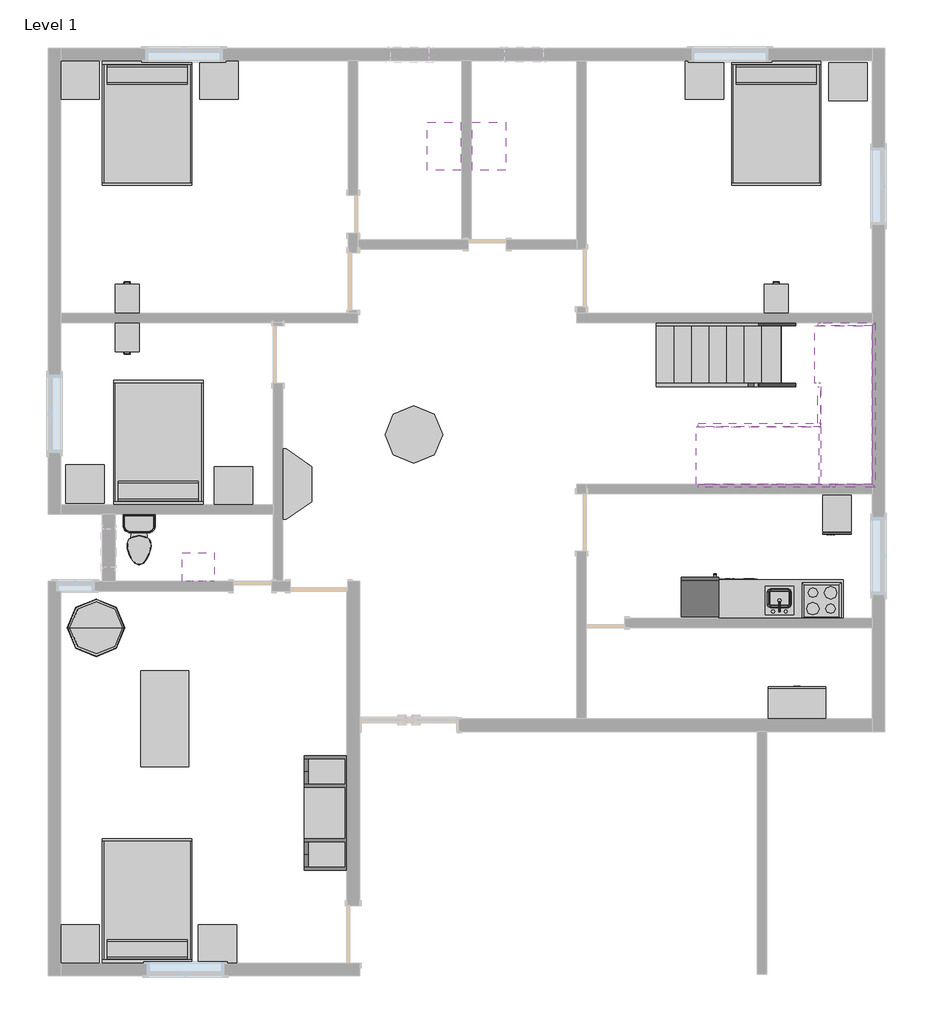
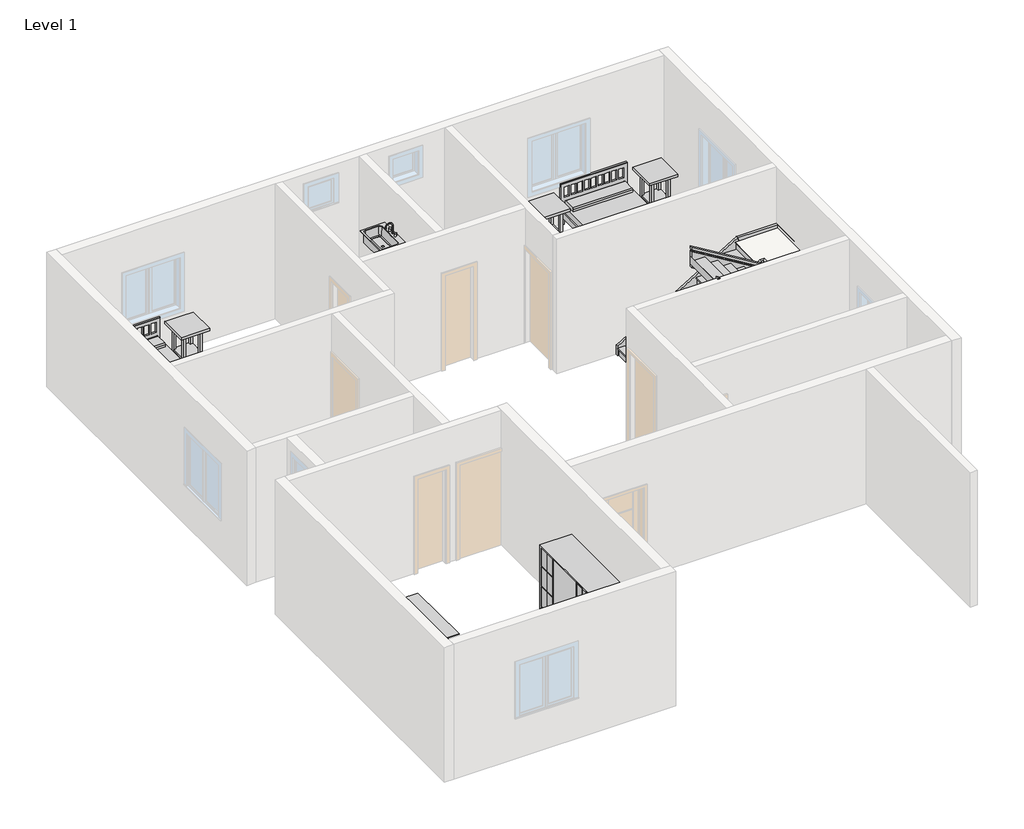
# One storey, part 2 of 2: 22 furniture elements, 8 members, 5 flow terminals, 5 proxies, 2 stair flights, 1 railing, 1 slab.
"""IFC4 building model written with IfcOpenShell, lengths in millimetres."""

from ifc_helpers import new_model, si_unit, frame, origin, place, context, project, spatial, polyline, outline, extrude, faceted_brep, transform, mapped, element, save
from components import proxy_7e1014cc, proxy_a6faaae8, proxy_45b28599, kitchenette_medium_kitchenette_medium_844211aa, proxy_c523a7b7, flow_terminal_98dee406, flow_terminal_871c2e40, flow_terminal_38af2918, toilet_domestic_3d_toilet_domestic_3d_f7549cf7, toilet_domestic_3d_toilet_domestic_3d_183bbd19, furniture_096e7f55, furniture_bb55ed6b, furniture_552c1472, furniture_c6510c7c, furniture_cf0b6580, furniture_e1dba61b, tv_stand_tv_stand_6ce107e5, furniture_37c8c8f5, furniture_905aceb5, furniture_5bc9ed15, furniture_c80d6d9c, non_monolithic_landing_c967b2c0, stair_flight_b85e79d8, stair_flight_81020766

model = new_model("IFC4")

# Units and contexts
model_context = context("Model", 3, world=origin())
ifc_project = project(units=[si_unit("LENGTHUNIT", "METRE", prefix="MILLI")], contexts=[model_context])

# Site, building, storey
site = spatial("IfcSite", under=ifc_project)
building = spatial("IfcBuilding", under=site)
storey = spatial("IfcBuildingStorey", under=building, Name="Level 1", Elevation=0.0)

# Proxies
placement = place(None, origin())
proxy_shape = proxy_7e1014cc(model_context)
element("IfcBuildingElementProxy", 1, Name="18\" x 24\" x 34 1/2\"", ObjectType="18\" x 24\" x 34 1/2\"", at=placement, inside=storey, context=model_context, shape_type="MappedRepresentation", body=[
    mapped(proxy_shape, transform((-3952.7899776, 8163.0653578, 0.0), x_axis=(1.0, 0.0, 0.0), y_axis=(0.0, 1.0, 0.0), z_axis=(0.0, 0.0, 1.0))),
])
proxy_2_shape = proxy_a6faaae8(model_context)
element("IfcBuildingElementProxy", 2, Name="Cook Top-4 Unit2 : 22\" x 20\"", ObjectType="Cook Top-4 Unit2 : 22\" x 20\"", at=placement, inside=storey, context=model_context, shape_type="MappedRepresentation", body=[
    mapped(proxy_2_shape, transform((-3887.9725091, 7057.9149226, 0.0), x_axis=(-1.0000000000000002, 0.0, 0.0), y_axis=(0.0, -1.0000000000000002, 0.0), z_axis=(0.0, 0.0, 1.0))),
])
proxy_3_shape = proxy_45b28599(model_context)
element("IfcBuildingElementProxy", 3, Name="Dishwasher : 24\" x 24\" x 34\"", ObjectType="Dishwasher : 24\" x 24\" x 34\"", at=placement, inside=storey, context=model_context, shape_type="MappedRepresentation", body=[
    mapped(proxy_3_shape, transform((-4839.1550406, 7349.7644874, 0.0), x_axis=(-1.0000000000000002, 0.0, 0.0), y_axis=(0.0, -1.0000000000000002, 0.0), z_axis=(0.0, 0.0, 1.0))),
])
kitchenette_medium_kitchenette_medium_shape = kitchenette_medium_kitchenette_medium_844211aa(model_context)
element("IfcBuildingElementProxy", 4, Name="Kitchenette - Medium : Kitchenette - Medium", ObjectType="Kitchenette - Medium : Kitchenette - Medium", at=placement, inside=storey, context=model_context, shape_type="MappedRepresentation", body=[
    mapped(kitchenette_medium_kitchenette_medium_shape, transform((-4212.1348042, 6753.1149226, 0.0), x_axis=(-1.0000000000000002, 0.0, 0.0), y_axis=(0.0, -1.0000000000000002, 0.0), z_axis=(0.0, 0.0, 1.0))),
])
proxy_4_shape = proxy_c523a7b7(model_context)
element("IfcBuildingElementProxy", 5, Name="Refrigerator : 24\" x 25\" LH", ObjectType="Refrigerator : 24\" x 25\" LH", at=placement, inside=storey, context=model_context, shape_type="MappedRepresentation", body=[
    mapped(proxy_4_shape, transform((-5824.7225091, 7103.5638941, 0.0), x_axis=(-1.0000000000000002, 0.0, 0.0), y_axis=(0.0, -1.0000000000000002, 0.0), z_axis=(0.0, 0.0, 1.0))),
])

# Flow terminals
flow_terminal_shape = flow_terminal_98dee406(model_context)
element("IfcFlowTerminal", 6, ObjectType="Sink - Work : 20\"x18\"", at=placement, inside=storey, context=model_context, shape_type="MappedRepresentation", body=[
    mapped(flow_terminal_shape, transform((-13806.6725091, 7362.7149226, 1524.0), x_axis=(-1.0000000000000004, 0.0, 0.0), y_axis=(0.0, -1.0000000000000004, 0.0), z_axis=(0.0, 0.0, 1.0))),
])
flow_terminal_2_shape = flow_terminal_871c2e40(model_context)
element("IfcFlowTerminal", 7, ObjectType="Sink Kitchen-Island : 18\" x 18\"", at=placement, inside=storey, context=model_context, shape_type="MappedRepresentation", body=[
    mapped(flow_terminal_2_shape, transform((-4545.3832686, 7060.2603237, -14.4), x_axis=(-1.0000000000000002, 0.0, 0.0), y_axis=(0.0, -1.0000000000000002, 0.0), z_axis=(0.0, 0.0, 1.0))),
])
flow_terminal_3_shape = flow_terminal_38af2918(model_context)
element("IfcFlowTerminal", 8, ObjectType="Sink Kitchen-Single : 30\" x 21\"", at=placement, inside=storey, context=model_context, shape_type="MappedRepresentation", body=[
    mapped(flow_terminal_3_shape, transform((-9897.4179102, 14299.9041632, 1219.2), x_axis=(0.0, -1.0000000000000007, 0.0), y_axis=(1.0000000000000007, 0.0, 0.0), z_axis=(0.0, 0.0, 1.0))),
])
element("IfcFlowTerminal", 9, ObjectType="Sink Kitchen-Single : 30\" x 21\"", at=placement, inside=storey, context=model_context, shape_type="MappedRepresentation", body=[
    mapped(flow_terminal_3_shape, transform((-9181.527108, 14268.5256821, 1219.2), x_axis=(0.0, 1.0, 0.0), y_axis=(-1.0, 0.0, 0.0), z_axis=(0.0, 0.0, 1.0))),
])
toilet_domestic_3d_toilet_domestic_3d_shape = toilet_domestic_3d_toilet_domestic_3d_f7549cf7(model_context)
toilet_domestic_3d_toilet_domestic_3d_2_shape = toilet_domestic_3d_toilet_domestic_3d_183bbd19(model_context)
element("IfcFlowTerminal", 10, ObjectType="Toilet-Domestic-3D : Toilet-Domestic-3D", at=placement, inside=storey, context=model_context, shape_type="MappedRepresentation", body=[
    mapped(toilet_domestic_3d_toilet_domestic_3d_shape, transform((-14746.4725091, 7934.8188953, 0.0), x_axis=(1.0, 0.0, 0.0), y_axis=(0.0, 1.0, 0.0), z_axis=(0.0, 0.0, 1.0))),
    mapped(toilet_domestic_3d_toilet_domestic_3d_2_shape, transform((-14746.4725091, 7934.8188953, 0.0), x_axis=(1.0, 0.0, 0.0), y_axis=(0.0, 1.0, 0.0), z_axis=(0.0, 0.0, 1.0))),
])

# Furniture
furniture_shape = furniture_096e7f55(model_context)
element("IfcFurniture", 11, ObjectType="Bed-Shaker : Double 56\" x 78\"", at=placement, inside=storey, context=model_context, shape_type="MappedRepresentation", body=[
    mapped(furniture_shape, transform((-4592.8225091, 15643.1149226, 0.0), x_axis=(1.0, 0.0, 0.0), y_axis=(0.0, 1.0, 0.0), z_axis=(0.0, 0.0, 1.0))),
])
element("IfcFurniture", 12, ObjectType="Bed-Shaker : Double 56\" x 78\"", at=placement, inside=storey, context=model_context, shape_type="MappedRepresentation", body=[
    mapped(furniture_shape, transform((-14600.4225091, 15643.1149226, 0.0), x_axis=(1.0, 0.0, 0.0), y_axis=(0.0, 1.0, 0.0), z_axis=(0.0, 0.0, 1.0))),
])
element("IfcFurniture", 13, ObjectType="Bed-Shaker : Double 56\" x 78\"", at=placement, inside=storey, context=model_context, shape_type="MappedRepresentation", body=[
    mapped(furniture_shape, transform((-14460.7225091, 8581.9149226, 0.0), x_axis=(-1.0, 0.0, 0.0), y_axis=(0.0, -1.0, 0.0), z_axis=(0.0, 0.0, 1.0))),
])
element("IfcFurniture", 14, ObjectType="Bed-Shaker : Double 56\" x 78\"", at=placement, inside=storey, context=model_context, shape_type="MappedRepresentation", body=[
    mapped(furniture_shape, transform((-14638.5225091, 1292.1149226, 0.0), x_axis=(-1.0, 0.0, 0.0), y_axis=(0.0, -1.0, 0.0), z_axis=(0.0, 0.0, 1.0))),
])
furniture_2_shape = furniture_bb55ed6b(model_context)
element("IfcFurniture", 15, ObjectType="Cabinet-File 2 Drawer : 15\" x 18\"", at=placement, inside=storey, context=model_context, shape_type="MappedRepresentation", body=[
    mapped(furniture_2_shape, transform((-14809.0760621, 11391.0492228, 0.0), x_axis=(1.0, 0.0, 0.0), y_axis=(0.0, 1.0, 0.0), z_axis=(0.0, 0.0, 1.0))),
])
furniture_3_shape = furniture_552c1472(model_context)
element("IfcFurniture", 16, ObjectType="Cabinet-File 3 Drawer : 15\" x 18\"", at=placement, inside=storey, context=model_context, shape_type="MappedRepresentation", body=[
    mapped(furniture_3_shape, transform((-15064.8689562, 11716.3806225, 0.0), x_axis=(-1.0000000000000004, 0.0, 0.0), y_axis=(0.0, -1.0000000000000004, 0.0), z_axis=(0.0, 0.0, 1.0))),
])
element("IfcFurniture", 17, ObjectType="Cabinet-File 3 Drawer : 15\" x 18\"", at=placement, inside=storey, context=model_context, shape_type="MappedRepresentation", body=[
    mapped(furniture_3_shape, transform((-4739.7689562, 11716.3806225, 0.0), x_axis=(-1.0000000000000004, 0.0, 0.0), y_axis=(0.0, -1.0000000000000004, 0.0), z_axis=(0.0, 0.0, 1.0))),
])
furniture_4_shape = furniture_c6510c7c(model_context)
element("IfcFurniture", 18, ObjectType="Counter Top w Sink Hole : 24\" Depth", at=placement, inside=storey, context=model_context, shape_type="MappedRepresentation", body=[
    mapped(furniture_4_shape, transform((-4745.5348042, 6753.1149226, -14.4), x_axis=(-1.0000000000000002, 0.0, 0.0), y_axis=(0.0, -1.0000000000000002, 0.0), z_axis=(0.0, 0.0, 1.0))),
])
furniture_5_shape = furniture_cf0b6580(model_context)
element("IfcFurniture", 19, ObjectType="Entertainment Center : 72\" x 72\" x 24\"", at=placement, inside=storey, context=model_context, shape_type="MappedRepresentation", body=[
    mapped(furniture_5_shape, transform((-11342.8725091, 3679.7149226, 0.0), x_axis=(0.0, -1.0000000000000004, 0.0), y_axis=(1.0000000000000004, 0.0, 0.0), z_axis=(0.0, 0.0, 1.0))),
])
furniture_6_shape = furniture_e1dba61b(model_context)
element("IfcFurniture", 20, ObjectType="Storage Pedestal : 20\" x 36\" x 36\"", at=placement, inside=storey, context=model_context, shape_type="MappedRepresentation", body=[
    mapped(furniture_6_shape, transform((-4461.6950231, 4497.9965466, 0.0), x_axis=(-1.0000000000000004, 0.0, 0.0), y_axis=(0.0, -1.0000000000000004, 0.0), z_axis=(0.0, 0.0, 1.0))),
])
tv_stand_tv_stand_shape = tv_stand_tv_stand_6ce107e5(model_context)
element("IfcFurniture", 21, ObjectType="TV Stand : TV Stand", at=placement, inside=storey, context=model_context, shape_type="MappedRepresentation", body=[
    mapped(tv_stand_tv_stand_shape, transform((-12003.2725091, 9037.3029247, 0.0), x_axis=(0.0, -1.000000000000001, 0.0), y_axis=(1.000000000000001, 0.0, 0.0), z_axis=(0.0, 0.0, 1.0))),
])
furniture_7_shape = furniture_37c8c8f5(model_context)
element("IfcFurniture", 22, ObjectType="Table-Dining : 30\" x 84\" x 22\"", at=placement, inside=storey, context=model_context, shape_type="MappedRepresentation", body=[
    mapped(furniture_7_shape, transform((-14244.8614313, 5160.049156, 0.0), x_axis=(0.0, 1.0, 0.0), y_axis=(-1.0, 0.0, 0.0), z_axis=(0.0, 0.0, 1.0))),
])
furniture_8_shape = furniture_905aceb5(model_context)
element("IfcFurniture", 23, ObjectType="Table-Dining Round w Chairs : 36\" Diameter", at=placement, inside=storey, context=model_context, shape_type="MappedRepresentation", body=[
    mapped(furniture_8_shape, transform((-10481.3544763, 9884.3936112, 0.0), x_axis=(1.0, 0.0, 0.0), y_axis=(0.0, 1.0, 0.0), z_axis=(0.0, 0.0, 1.0))),
])
furniture_9_shape = furniture_5bc9ed15(model_context)
element("IfcFurniture", 24, ObjectType="Table-Night Stand : 24\" x 24\" x 30\"", at=placement, inside=storey, context=model_context, shape_type="MappedRepresentation", body=[
    mapped(furniture_9_shape, transform((-15994.8061394, 1292.1149226, 0.0), x_axis=(1.0, 0.0, 0.0), y_axis=(0.0, 1.0, 0.0), z_axis=(0.0, 0.0, 1.0))),
])
element("IfcFurniture", 25, ObjectType="Table-Night Stand : 24\" x 24\" x 30\"", at=placement, inside=storey, context=model_context, shape_type="MappedRepresentation", body=[
    mapped(furniture_9_shape, transform((-13810.4061394, 1292.1149226, 0.0), x_axis=(1.0, 0.0, 0.0), y_axis=(0.0, 1.0, 0.0), z_axis=(0.0, 0.0, 1.0))),
])
element("IfcFurniture", 26, ObjectType="Table-Night Stand : 24\" x 24\" x 30\"", at=placement, inside=storey, context=model_context, shape_type="MappedRepresentation", body=[
    mapped(furniture_9_shape, transform((-15918.6061394, 8607.3149226, 0.0), x_axis=(1.0, 0.0, 0.0), y_axis=(0.0, 1.0, 0.0), z_axis=(0.0, 0.0, 1.0))),
])
element("IfcFurniture", 27, ObjectType="Table-Night Stand : 24\" x 24\" x 30\"", at=placement, inside=storey, context=model_context, shape_type="MappedRepresentation", body=[
    mapped(furniture_9_shape, transform((-13556.4061394, 8581.9149226, 0.0), x_axis=(1.0, 0.0, 0.0), y_axis=(0.0, 1.0, 0.0), z_axis=(0.0, 0.0, 1.0))),
])
element("IfcFurniture", 28, ObjectType="Table-Night Stand : 24\" x 24\" x 30\"", at=placement, inside=storey, context=model_context, shape_type="MappedRepresentation", body=[
    mapped(furniture_9_shape, transform((-15994.8061394, 15033.5149226, 0.0), x_axis=(1.0, 0.0, 0.0), y_axis=(0.0, 1.0, 0.0), z_axis=(0.0, 0.0, 1.0))),
])
element("IfcFurniture", 29, ObjectType="Table-Night Stand : 24\" x 24\" x 30\"", at=placement, inside=storey, context=model_context, shape_type="MappedRepresentation", body=[
    mapped(furniture_9_shape, transform((-13785.0061394, 15033.5149226, 0.0), x_axis=(1.0, 0.0, 0.0), y_axis=(0.0, 1.0, 0.0), z_axis=(0.0, 0.0, 1.0))),
])
element("IfcFurniture", 30, ObjectType="Table-Night Stand : 24\" x 24\" x 30\"", at=placement, inside=storey, context=model_context, shape_type="MappedRepresentation", body=[
    mapped(furniture_9_shape, transform((-6063.4061394, 15033.5149226, 0.0), x_axis=(1.0, 0.0, 0.0), y_axis=(0.0, 1.0, 0.0), z_axis=(0.0, 0.0, 1.0))),
])
element("IfcFurniture", 31, ObjectType="Table-Night Stand : 24\" x 24\" x 30\"", at=placement, inside=storey, context=model_context, shape_type="MappedRepresentation", body=[
    mapped(furniture_9_shape, transform((-3777.4061394, 15008.1149226, 0.0), x_axis=(1.0, 0.0, 0.0), y_axis=(0.0, 1.0, 0.0), z_axis=(0.0, 0.0, 1.0))),
])
furniture_10_shape = furniture_c80d6d9c(model_context)
element("IfcFurniture", 32, ObjectType="Table-Round : 36\" Diameter", at=placement, inside=storey, context=model_context, shape_type="MappedRepresentation", body=[
    mapped(furniture_10_shape, transform((-15432.2725091, 6626.1149226, 0.0), x_axis=(1.0, 0.0, 0.0), y_axis=(0.0, 1.0, 0.0), z_axis=(0.0, 0.0, 1.0))),
])

# Members
element("IfcMember", 33, ObjectType="Stringer - 2\" Width", at=placement, inside=storey, context=model_context, shape_type="SweptSolid", body=[
    extrude(outline(polyline([(212.114512, -6516.8725091), (0.0, -6516.8725091), (0.0, -6278.7869974), (1464.7333333, -3861.9769974), (1769.5333333, -3947.1314539), (212.114512, -6516.8725091)])), frame((0.0, 11426.7149226, 0.0), z_axis=(0.0, 1.0, 0.0), x_axis=(0.0, 0.0, 1.0)), (0.0, 0.0, 1.0), 50.8),
])
element("IfcMember", 34, ObjectType="Stringer - 2\" Width", at=placement, inside=storey, context=model_context, shape_type="SweptSolid", body=[
    extrude(outline(polyline([(212.114512, -6516.8725091), (0.0, -6516.8725091), (0.0, -6278.7869974), (1441.281508, -3900.6725091), (1769.5333333, -3900.6725091), (1769.5333333, -3947.1314539), (212.114512, -6516.8725091)])), frame((0.0, 10461.5149226, 0.0), z_axis=(0.0, 1.0, 0.0), x_axis=(0.0, 0.0, 1.0)), (0.0, 0.0, 1.0), 50.8),
])
element("IfcMember", 35, ObjectType="Stringer - 2\" Width", at=placement, inside=storey, context=model_context, shape_type="SweptSolid", body=[
    extrude(outline(polyline([(1464.7333333, -3761.5680209), (1769.5333333, -3676.4135644), (3090.7811786, -5856.4725091), (2734.3724171, -5856.4725091), (1464.7333333, -3761.5680209)])), frame((0.0, 8861.3149226, 0.0), z_axis=(0.0, 1.0, 0.0), x_axis=(0.0, 0.0, 1.0)), (0.0, 0.0, 1.0), 50.8),
])
element("IfcMember", 36, ObjectType="Stringer - 2\" Width", at=placement, inside=storey, context=model_context, shape_type="SweptSolid", body=[
    extrude(outline(polyline([(1549.0390838, -3900.6725091), (1905.4478453, -3900.6725091), (3090.7811786, -5856.4725091), (2734.3724171, -5856.4725091), (1549.0390838, -3900.6725091)])), frame((0.0, 9826.5149226, 0.0), z_axis=(0.0, 1.0, 0.0), x_axis=(0.0, 0.0, 1.0)), (0.0, 0.0, 1.0), 50.8),
])
element("IfcMember", 37, ObjectType="Stringer - 2\" Width", at=placement, inside=storey, context=model_context, shape_type="Brep", body=[
    faceted_brep([(-3676.4135644, 8912.1149226, 1769.5333333), (-3676.4135644, 8861.3149226, 1769.5333333), (-3037.0725091, 8861.3149226, 1769.5333333), (-3087.8725091, 8912.1149226, 1769.5333333), (-3761.5680209, 8912.1149226, 1464.7333333), (-3087.8725091, 8912.1149226, 1464.7333333), (-3761.5680209, 8861.3149226, 1464.7333333), (-3037.0725091, 8861.3149226, 1464.7333333)], [[[0, 1, 2, 3]], [[4, 0, 3, 5]], [[6, 4, 5, 7]], [[1, 6, 7, 2]], [[1, 0, 4, 6]], [[2, 7, 5, 3]]]),
])
element("IfcMember", 38, ObjectType="Stringer - 2\" Width", at=placement, inside=storey, context=model_context, shape_type="SweptSolid", body=[
    extrude(outline(polyline([(-3037.0725091, 8861.3149226), (-3087.8725091, 8912.1149226), (-3087.8725091, 11426.7149226), (-3037.0725091, 11477.5149226), (-3037.0725091, 8861.3149226)])), frame((0.0, 0.0, 1464.7333333), z_axis=(0.0, 0.0, 1.0), x_axis=(1.0, 0.0, 0.0)), (0.0, 0.0, 1.0), 304.8),
])
element("IfcMember", 39, ObjectType="Stringer - 2\" Width", at=placement, inside=storey, context=model_context, shape_type="Brep", body=[
    faceted_brep([(-3087.8725091, 11426.7149226, 1769.5333333), (-3037.0725091, 11477.5149226, 1769.5333333), (-3947.1314539, 11477.5149226, 1769.5333333), (-3947.1314539, 11426.7149226, 1769.5333333), (-3087.8725091, 11426.7149226, 1464.7333333), (-3861.9769974, 11426.7149226, 1464.7333333), (-3037.0725091, 11477.5149226, 1464.7333333), (-3861.9769974, 11477.5149226, 1464.7333333)], [[[0, 1, 2, 3]], [[4, 0, 3, 5]], [[6, 4, 5, 7]], [[1, 6, 7, 2]], [[1, 0, 4, 6]], [[2, 7, 5, 3]]]),
])
element("IfcMember", 40, ObjectType="Stringer - 2\" Width", at=placement, inside=storey, context=model_context, shape_type="SweptSolid", body=[
    extrude(outline(polyline([(-3951.4725091, 10461.5149226), (-3900.6725091, 10461.5149226), (-3900.6725091, 9877.3149226), (-3951.4725091, 9877.3149226), (-3951.4725091, 10461.5149226)])), frame((0.0, 0.0, 1464.7333333), z_axis=(0.0, 0.0, 1.0), x_axis=(1.0, 0.0, 0.0)), (0.0, 0.0, 1.0), 304.8),
])

# Railing
element("IfcRailing", 41, ObjectType="Handrail - Rectangular", at=placement, inside=storey, context=model_context, shape_type="SolidModel", body=[
    faceted_brep([(-6516.8725091, 10512.3149226, 321.7333333), (-6516.8725091, 10512.3149226, 262.3318731), (-6516.8725091, 10461.5149226, 262.3318731), (-6516.8725091, 10461.5149226, 321.7333333), (-4002.2725091, 10512.3149226, 1845.7333333), (-3988.0800997, 10512.3149226, 1794.9333333), (-3988.0800997, 10461.5149226, 1794.9333333), (-4002.2725091, 10461.5149226, 1845.7333333), (-3900.6725091, 10512.3149226, 1845.7333333), (-3900.6725091, 10512.3149226, 1794.9333333), (-3951.4725091, 10461.5149226, 1794.9333333), (-3951.4725091, 10461.5149226, 1845.7333333), (-3900.6725091, 9953.5149226, 1845.7333333), (-3900.6725091, 9902.7149226, 1794.9333333), (-3951.4725091, 9902.7149226, 1794.9333333), (-3951.4725091, 9953.5149226, 1845.7333333), (-3900.6725091, 9953.5149226, 2092.0363636), (-3900.6725091, 9902.7149226, 2041.2363636), (-3951.4725091, 9902.7149226, 2041.2363636), (-3951.4725091, 9953.5149226, 2092.0363636), (-3900.6725091, 9826.5149226, 2092.0363636), (-3900.6725091, 9826.5149226, 2041.2363636), (-3951.4725091, 9877.3149226, 2041.2363636), (-3951.4725091, 9877.3149226, 2092.0363636), (-4027.6725091, 9826.5149226, 2092.0363636), (-4041.8649185, 9826.5149226, 2041.2363636), (-4041.8649185, 9877.3149226, 2041.2363636), (-4027.6725091, 9877.3149226, 2092.0363636), (-5856.4725091, 9826.5149226, 3200.4), (-5856.4725091, 9877.3149226, 3200.4), (-5856.4725091, 9877.3149226, 3140.9985397), (-5856.4725091, 9826.5149226, 3140.9985397)], [[[0, 1, 2, 3]], [[1, 0, 4, 5]], [[2, 1, 5, 6]], [[3, 2, 6, 7]], [[0, 3, 7, 4]], [[5, 4, 8, 9]], [[6, 5, 9, 10]], [[7, 6, 10, 11]], [[4, 7, 11, 8]], [[9, 8, 12, 13]], [[10, 9, 13, 14]], [[11, 10, 14, 15]], [[8, 11, 15, 12]], [[13, 12, 16, 17]], [[14, 13, 17, 18]], [[15, 14, 18, 19]], [[12, 15, 19, 16]], [[17, 16, 20, 21]], [[18, 17, 21, 22]], [[19, 18, 22, 23]], [[16, 19, 23, 20]], [[21, 20, 24, 25]], [[22, 21, 25, 26]], [[23, 22, 26, 27]], [[20, 23, 27, 24]], [[28, 29, 30, 31]], [[25, 24, 28, 31]], [[26, 25, 31, 30]], [[27, 26, 30, 29]], [[24, 27, 29, 28]]]),
    extrude(outline(polyline([(3073.6500549, -5745.3475091), (3085.1955094, -5764.3975091), (3034.9781483, -5764.3975091), (3023.4326938, -5745.3475091), (3073.6500549, -5745.3475091)])), frame((0.0, 9842.3899226, 0.0), z_axis=(0.0, 1.0, 0.0), x_axis=(0.0, 0.0, 1.0)), (0.0, 0.0, 1.0), 19.05),
    extrude(outline(polyline([(3012.0742973, -5643.7475091), (3023.6197519, -5662.7975091), (2973.4023907, -5662.7975091), (2961.8569362, -5643.7475091), (3012.0742973, -5643.7475091)])), frame((0.0, 9842.3899226, 0.0), z_axis=(0.0, 1.0, 0.0), x_axis=(0.0, 0.0, 1.0)), (0.0, 0.0, 1.0), 19.05),
    extrude(outline(polyline([(2950.4985397, -5542.1475091), (2962.0439943, -5561.1975091), (2911.8266332, -5561.1975091), (2900.2811786, -5542.1475091), (2950.4985397, -5542.1475091)])), frame((0.0, 9842.3899226, 0.0), z_axis=(0.0, 1.0, 0.0), x_axis=(0.0, 0.0, 1.0)), (0.0, 0.0, 1.0), 19.05),
    extrude(outline(polyline([(2888.9227822, -5440.5475091), (2900.4682367, -5459.5975091), (2850.2508756, -5459.5975091), (2838.7054211, -5440.5475091), (2888.9227822, -5440.5475091)])), frame((0.0, 9842.3899226, 0.0), z_axis=(0.0, 1.0, 0.0), x_axis=(0.0, 0.0, 1.0)), (0.0, 0.0, 1.0), 19.05),
    extrude(outline(polyline([(2827.3470246, -5338.9475091), (2838.8924791, -5357.9975091), (2788.675118, -5357.9975091), (2777.1296635, -5338.9475091), (2827.3470246, -5338.9475091)])), frame((0.0, 9842.3899226, 0.0), z_axis=(0.0, 1.0, 0.0), x_axis=(0.0, 0.0, 1.0)), (0.0, 0.0, 1.0), 19.05),
    extrude(outline(polyline([(2765.771267, -5237.3475091), (2777.3167216, -5256.3975091), (2727.0993604, -5256.3975091), (2715.5539059, -5237.3475091), (2765.771267, -5237.3475091)])), frame((0.0, 9842.3899226, 0.0), z_axis=(0.0, 1.0, 0.0), x_axis=(0.0, 0.0, 1.0)), (0.0, 0.0, 1.0), 19.05),
    extrude(outline(polyline([(2704.1955094, -5135.7475091), (2715.740964, -5154.7975091), (2665.5236029, -5154.7975091), (2653.9781483, -5135.7475091), (2704.1955094, -5135.7475091)])), frame((0.0, 9842.3899226, 0.0), z_axis=(0.0, 1.0, 0.0), x_axis=(0.0, 0.0, 1.0)), (0.0, 0.0, 1.0), 19.05),
    extrude(outline(polyline([(2642.6197519, -5034.1475091), (2654.1652064, -5053.1975091), (2603.9478453, -5053.1975091), (2592.4023907, -5034.1475091), (2642.6197519, -5034.1475091)])), frame((0.0, 9842.3899226, 0.0), z_axis=(0.0, 1.0, 0.0), x_axis=(0.0, 0.0, 1.0)), (0.0, 0.0, 1.0), 19.05),
    extrude(outline(polyline([(2581.0439943, -4932.5475091), (2592.5894488, -4951.5975091), (2542.3720877, -4951.5975091), (2530.8266332, -4932.5475091), (2581.0439943, -4932.5475091)])), frame((0.0, 9842.3899226, 0.0), z_axis=(0.0, 1.0, 0.0), x_axis=(0.0, 0.0, 1.0)), (0.0, 0.0, 1.0), 19.05),
    extrude(outline(polyline([(2519.4682367, -4830.9475091), (2531.0136913, -4849.9975091), (2480.7963301, -4849.9975091), (2469.2508756, -4830.9475091), (2519.4682367, -4830.9475091)])), frame((0.0, 9842.3899226, 0.0), z_axis=(0.0, 1.0, 0.0), x_axis=(0.0, 0.0, 1.0)), (0.0, 0.0, 1.0), 19.05),
    extrude(outline(polyline([(2457.8924791, -4729.3475091), (2469.4379337, -4748.3975091), (2419.2205726, -4748.3975091), (2407.675118, -4729.3475091), (2457.8924791, -4729.3475091)])), frame((0.0, 9842.3899226, 0.0), z_axis=(0.0, 1.0, 0.0), x_axis=(0.0, 0.0, 1.0)), (0.0, 0.0, 1.0), 19.05),
    extrude(outline(polyline([(2396.3167216, -4627.7475091), (2407.8621761, -4646.7975091), (2357.644815, -4646.7975091), (2346.0993604, -4627.7475091), (2396.3167216, -4627.7475091)])), frame((0.0, 9842.3899226, 0.0), z_axis=(0.0, 1.0, 0.0), x_axis=(0.0, 0.0, 1.0)), (0.0, 0.0, 1.0), 19.05),
    extrude(outline(polyline([(2334.740964, -4526.1475091), (2346.2864185, -4545.1975091), (2296.0690574, -4545.1975091), (2284.5236029, -4526.1475091), (2334.740964, -4526.1475091)])), frame((0.0, 9842.3899226, 0.0), z_axis=(0.0, 1.0, 0.0), x_axis=(0.0, 0.0, 1.0)), (0.0, 0.0, 1.0), 19.05),
    extrude(outline(polyline([(2273.1652064, -4424.5475091), (2284.710661, -4443.5975091), (2234.4932998, -4443.5975091), (2222.9478453, -4424.5475091), (2273.1652064, -4424.5475091)])), frame((0.0, 9842.3899226, 0.0), z_axis=(0.0, 1.0, 0.0), x_axis=(0.0, 0.0, 1.0)), (0.0, 0.0, 1.0), 19.05),
    extrude(outline(polyline([(2211.5894488, -4322.9475091), (2223.1349034, -4341.9975091), (2172.9175423, -4341.9975091), (2161.3720877, -4322.9475091), (2211.5894488, -4322.9475091)])), frame((0.0, 9842.3899226, 0.0), z_axis=(0.0, 1.0, 0.0), x_axis=(0.0, 0.0, 1.0)), (0.0, 0.0, 1.0), 19.05),
    extrude(outline(polyline([(2150.0136913, -4221.3475091), (2161.5591458, -4240.3975091), (2111.3417847, -4240.3975091), (2099.7963301, -4221.3475091), (2150.0136913, -4221.3475091)])), frame((0.0, 9842.3899226, 0.0), z_axis=(0.0, 1.0, 0.0), x_axis=(0.0, 0.0, 1.0)), (0.0, 0.0, 1.0), 19.05),
    extrude(outline(polyline([(2088.4379337, -4119.7475091), (2099.9833882, -4138.7975091), (2049.7660271, -4138.7975091), (2038.2205726, -4119.7475091), (2088.4379337, -4119.7475091)])), frame((0.0, 9842.3899226, 0.0), z_axis=(0.0, 1.0, 0.0), x_axis=(0.0, 0.0, 1.0)), (0.0, 0.0, 1.0), 19.05),
    extrude(outline(polyline([(2041.2363636, -4018.1475091), (2041.2363636, -4037.1975091), (1988.1902695, -4037.1975091), (1976.644815, -4018.1475091), (2041.2363636, -4018.1475091)])), frame((0.0, 9842.3899226, 0.0), z_axis=(0.0, 1.0, 0.0), x_axis=(0.0, 0.0, 1.0)), (0.0, 0.0, 1.0), 19.05),
    extrude(outline(polyline([(-3935.5975091, 9886.8399226), (-3916.5475091, 9886.8399226), (-3916.5475091, 9867.7899226), (-3935.5975091, 9867.7899226), (-3935.5975091, 9886.8399226)])), frame((0.0, 0.0, 1769.5333333), z_axis=(0.0, 0.0, 1.0), x_axis=(1.0, 0.0, 0.0)), (0.0, 0.0, 1.0), 25.4),
    extrude(outline(polyline([(-3935.5975091, 9988.4399226), (-3916.5475091, 9988.4399226), (-3916.5475091, 9969.3899226), (-3935.5975091, 9969.3899226), (-3935.5975091, 9988.4399226)])), frame((0.0, 0.0, 1769.5333333), z_axis=(0.0, 0.0, 1.0), x_axis=(1.0, 0.0, 0.0)), (0.0, 0.0, 1.0), 25.4),
    extrude(outline(polyline([(-3935.5975091, 10090.0399226), (-3916.5475091, 10090.0399226), (-3916.5475091, 10070.9899226), (-3935.5975091, 10070.9899226), (-3935.5975091, 10090.0399226)])), frame((0.0, 0.0, 1769.5333333), z_axis=(0.0, 0.0, 1.0), x_axis=(1.0, 0.0, 0.0)), (0.0, 0.0, 1.0), 25.4),
    extrude(outline(polyline([(-3935.5975091, 10191.6399226), (-3916.5475091, 10191.6399226), (-3916.5475091, 10172.5899226), (-3935.5975091, 10172.5899226), (-3935.5975091, 10191.6399226)])), frame((0.0, 0.0, 1769.5333333), z_axis=(0.0, 0.0, 1.0), x_axis=(1.0, 0.0, 0.0)), (0.0, 0.0, 1.0), 25.4),
    extrude(outline(polyline([(-3935.5975091, 10293.2399226), (-3916.5475091, 10293.2399226), (-3916.5475091, 10274.1899226), (-3935.5975091, 10274.1899226), (-3935.5975091, 10293.2399226)])), frame((0.0, 0.0, 1769.5333333), z_axis=(0.0, 0.0, 1.0), x_axis=(1.0, 0.0, 0.0)), (0.0, 0.0, 1.0), 25.4),
    extrude(outline(polyline([(-3935.5975091, 10394.8399226), (-3916.5475091, 10394.8399226), (-3916.5475091, 10375.7899226), (-3935.5975091, 10375.7899226), (-3935.5975091, 10394.8399226)])), frame((0.0, 0.0, 1769.5333333), z_axis=(0.0, 0.0, 1.0), x_axis=(1.0, 0.0, 0.0)), (0.0, 0.0, 1.0), 25.4),
    extrude(outline(polyline([(1745.9227822, -4068.9475091), (1734.3773276, -4087.9975091), (1684.1599665, -4087.9975091), (1695.7054211, -4068.9475091), (1745.9227822, -4068.9475091)])), frame((0.0, 10477.3899226, 0.0), z_axis=(0.0, 1.0, 0.0), x_axis=(0.0, 0.0, 1.0)), (0.0, 0.0, 1.0), 19.05),
    extrude(outline(polyline([(1684.3470246, -4170.5475091), (1672.80157, -4189.5975091), (1622.5842089, -4189.5975091), (1634.1296635, -4170.5475091), (1684.3470246, -4170.5475091)])), frame((0.0, 10477.3899226, 0.0), z_axis=(0.0, 1.0, 0.0), x_axis=(0.0, 0.0, 1.0)), (0.0, 0.0, 1.0), 19.05),
    extrude(outline(polyline([(1622.771267, -4272.1475091), (1611.2258125, -4291.1975091), (1561.0084514, -4291.1975091), (1572.5539059, -4272.1475091), (1622.771267, -4272.1475091)])), frame((0.0, 10477.3899226, 0.0), z_axis=(0.0, 1.0, 0.0), x_axis=(0.0, 0.0, 1.0)), (0.0, 0.0, 1.0), 19.05),
    extrude(outline(polyline([(1561.1955094, -4373.7475091), (1549.6500549, -4392.7975091), (1499.4326938, -4392.7975091), (1510.9781483, -4373.7475091), (1561.1955094, -4373.7475091)])), frame((0.0, 10477.3899226, 0.0), z_axis=(0.0, 1.0, 0.0), x_axis=(0.0, 0.0, 1.0)), (0.0, 0.0, 1.0), 19.05),
    extrude(outline(polyline([(1499.6197519, -4475.3475091), (1488.0742973, -4494.3975091), (1437.8569362, -4494.3975091), (1449.4023907, -4475.3475091), (1499.6197519, -4475.3475091)])), frame((0.0, 10477.3899226, 0.0), z_axis=(0.0, 1.0, 0.0), x_axis=(0.0, 0.0, 1.0)), (0.0, 0.0, 1.0), 19.05),
    extrude(outline(polyline([(1438.0439943, -4576.9475091), (1426.4985397, -4595.9975091), (1376.2811786, -4595.9975091), (1387.8266332, -4576.9475091), (1438.0439943, -4576.9475091)])), frame((0.0, 10477.3899226, 0.0), z_axis=(0.0, 1.0, 0.0), x_axis=(0.0, 0.0, 1.0)), (0.0, 0.0, 1.0), 19.05),
    extrude(outline(polyline([(1376.4682367, -4678.5475091), (1364.9227822, -4697.5975091), (1314.7054211, -4697.5975091), (1326.2508756, -4678.5475091), (1376.4682367, -4678.5475091)])), frame((0.0, 10477.3899226, 0.0), z_axis=(0.0, 1.0, 0.0), x_axis=(0.0, 0.0, 1.0)), (0.0, 0.0, 1.0), 19.05),
    extrude(outline(polyline([(1314.8924791, -4780.1475091), (1303.3470246, -4799.1975091), (1253.1296635, -4799.1975091), (1264.675118, -4780.1475091), (1314.8924791, -4780.1475091)])), frame((0.0, 10477.3899226, 0.0), z_axis=(0.0, 1.0, 0.0), x_axis=(0.0, 0.0, 1.0)), (0.0, 0.0, 1.0), 19.05),
    extrude(outline(polyline([(1253.3167216, -4881.7475091), (1241.771267, -4900.7975091), (1191.5539059, -4900.7975091), (1203.0993604, -4881.7475091), (1253.3167216, -4881.7475091)])), frame((0.0, 10477.3899226, 0.0), z_axis=(0.0, 1.0, 0.0), x_axis=(0.0, 0.0, 1.0)), (0.0, 0.0, 1.0), 19.05),
    extrude(outline(polyline([(1191.740964, -4983.3475091), (1180.1955094, -5002.3975091), (1129.9781483, -5002.3975091), (1141.5236029, -4983.3475091), (1191.740964, -4983.3475091)])), frame((0.0, 10477.3899226, 0.0), z_axis=(0.0, 1.0, 0.0), x_axis=(0.0, 0.0, 1.0)), (0.0, 0.0, 1.0), 19.05),
    extrude(outline(polyline([(1130.1652064, -5084.9475091), (1118.6197519, -5103.9975091), (1068.4023907, -5103.9975091), (1079.9478453, -5084.9475091), (1130.1652064, -5084.9475091)])), frame((0.0, 10477.3899226, 0.0), z_axis=(0.0, 1.0, 0.0), x_axis=(0.0, 0.0, 1.0)), (0.0, 0.0, 1.0), 19.05),
    extrude(outline(polyline([(1068.5894488, -5186.5475091), (1057.0439943, -5205.5975091), (1006.8266332, -5205.5975091), (1018.3720877, -5186.5475091), (1068.5894488, -5186.5475091)])), frame((0.0, 10477.3899226, 0.0), z_axis=(0.0, 1.0, 0.0), x_axis=(0.0, 0.0, 1.0)), (0.0, 0.0, 1.0), 19.05),
    extrude(outline(polyline([(1007.0136913, -5288.1475091), (995.4682367, -5307.1975091), (945.2508756, -5307.1975091), (956.7963301, -5288.1475091), (1007.0136913, -5288.1475091)])), frame((0.0, 10477.3899226, 0.0), z_axis=(0.0, 1.0, 0.0), x_axis=(0.0, 0.0, 1.0)), (0.0, 0.0, 1.0), 19.05),
    extrude(outline(polyline([(945.4379337, -5389.7475091), (933.8924791, -5408.7975091), (883.675118, -5408.7975091), (895.2205726, -5389.7475091), (945.4379337, -5389.7475091)])), frame((0.0, 10477.3899226, 0.0), z_axis=(0.0, 1.0, 0.0), x_axis=(0.0, 0.0, 1.0)), (0.0, 0.0, 1.0), 19.05),
    extrude(outline(polyline([(883.8621761, -5491.3475091), (872.3167216, -5510.3975091), (822.0993604, -5510.3975091), (833.644815, -5491.3475091), (883.8621761, -5491.3475091)])), frame((0.0, 10477.3899226, 0.0), z_axis=(0.0, 1.0, 0.0), x_axis=(0.0, 0.0, 1.0)), (0.0, 0.0, 1.0), 19.05),
    extrude(outline(polyline([(822.2864185, -5592.9475091), (810.740964, -5611.9975091), (760.5236029, -5611.9975091), (772.0690574, -5592.9475091), (822.2864185, -5592.9475091)])), frame((0.0, 10477.3899226, 0.0), z_axis=(0.0, 1.0, 0.0), x_axis=(0.0, 0.0, 1.0)), (0.0, 0.0, 1.0), 19.05),
    extrude(outline(polyline([(760.710661, -5694.5475091), (749.1652064, -5713.5975091), (698.9478453, -5713.5975091), (710.4932998, -5694.5475091), (760.710661, -5694.5475091)])), frame((0.0, 10477.3899226, 0.0), z_axis=(0.0, 1.0, 0.0), x_axis=(0.0, 0.0, 1.0)), (0.0, 0.0, 1.0), 19.05),
    extrude(outline(polyline([(699.1349034, -5796.1475091), (687.5894488, -5815.1975091), (637.3720877, -5815.1975091), (648.9175423, -5796.1475091), (699.1349034, -5796.1475091)])), frame((0.0, 10477.3899226, 0.0), z_axis=(0.0, 1.0, 0.0), x_axis=(0.0, 0.0, 1.0)), (0.0, 0.0, 1.0), 19.05),
    extrude(outline(polyline([(637.5591458, -5897.7475091), (626.0136913, -5916.7975091), (575.7963301, -5916.7975091), (587.3417847, -5897.7475091), (637.5591458, -5897.7475091)])), frame((0.0, 10477.3899226, 0.0), z_axis=(0.0, 1.0, 0.0), x_axis=(0.0, 0.0, 1.0)), (0.0, 0.0, 1.0), 19.05),
    extrude(outline(polyline([(575.9833882, -5999.3475091), (564.4379337, -6018.3975091), (514.2205726, -6018.3975091), (525.7660271, -5999.3475091), (575.9833882, -5999.3475091)])), frame((0.0, 10477.3899226, 0.0), z_axis=(0.0, 1.0, 0.0), x_axis=(0.0, 0.0, 1.0)), (0.0, 0.0, 1.0), 19.05),
    extrude(outline(polyline([(514.4076307, -6100.9475091), (502.8621761, -6119.9975091), (452.644815, -6119.9975091), (464.1902695, -6100.9475091), (514.4076307, -6100.9475091)])), frame((0.0, 10477.3899226, 0.0), z_axis=(0.0, 1.0, 0.0), x_axis=(0.0, 0.0, 1.0)), (0.0, 0.0, 1.0), 19.05),
    extrude(outline(polyline([(452.8318731, -6202.5475091), (441.2864185, -6221.5975091), (391.0690574, -6221.5975091), (402.614512, -6202.5475091), (452.8318731, -6202.5475091)])), frame((0.0, 10477.3899226, 0.0), z_axis=(0.0, 1.0, 0.0), x_axis=(0.0, 0.0, 1.0)), (0.0, 0.0, 1.0), 19.05),
    extrude(outline(polyline([(391.2561155, -6304.1475091), (379.710661, -6323.1975091), (329.4932998, -6323.1975091), (341.0387544, -6304.1475091), (391.2561155, -6304.1475091)])), frame((0.0, 10477.3899226, 0.0), z_axis=(0.0, 1.0, 0.0), x_axis=(0.0, 0.0, 1.0)), (0.0, 0.0, 1.0), 19.05),
    extrude(outline(polyline([(329.6803579, -6405.7475091), (318.1349034, -6424.7975091), (267.9175423, -6424.7975091), (279.4629968, -6405.7475091), (329.6803579, -6405.7475091)])), frame((0.0, 10477.3899226, 0.0), z_axis=(0.0, 1.0, 0.0), x_axis=(0.0, 0.0, 1.0)), (0.0, 0.0, 1.0), 19.05),
    extrude(outline(polyline([(-3916.5475091, 9861.4399226), (-3916.5475091, 9842.3899226), (-3935.5975091, 9842.3899226), (-3935.5975091, 9861.4399226), (-3916.5475091, 9861.4399226)])), frame((0.0, 0.0, 1693.3333333), z_axis=(0.0, 0.0, 1.0), x_axis=(1.0, 0.0, 0.0)), (0.0, 0.0, 1.0), 347.9030303),
    extrude(outline(polyline([(-3935.5975091, 10477.3899226), (-3935.5975091, 10496.4399226), (-3916.5475091, 10496.4399226), (-3916.5475091, 10477.3899226), (-3935.5975091, 10477.3899226)])), frame((0.0, 0.0, 1769.5333333), z_axis=(0.0, 0.0, 1.0), x_axis=(1.0, 0.0, 0.0)), (0.0, 0.0, 1.0), 25.4),
    extrude(outline(polyline([(1792.1046004, -3992.7475091), (1780.5591458, -4011.7975091), (1730.3417847, -4011.7975091), (1741.8872392, -3992.7475091), (1792.1046004, -3992.7475091)])), frame((0.0, 10477.3899226, 0.0), z_axis=(0.0, 1.0, 0.0), x_axis=(0.0, 0.0, 1.0)), (0.0, 0.0, 1.0), 19.05),
    extrude(outline(polyline([(3129.4530852, -5837.4225091), (3140.9985397, -5856.4725091), (3090.7811786, -5856.4725091), (3079.2357241, -5837.4225091), (3129.4530852, -5837.4225091)])), frame((0.0, 9842.3899226, 0.0), z_axis=(0.0, 1.0, 0.0), x_axis=(0.0, 0.0, 1.0)), (0.0, 0.0, 1.0), 19.05),
    extrude(outline(polyline([(273.8773276, -6497.8225091), (262.3318731, -6516.8725091), (212.114512, -6516.8725091), (223.6599665, -6497.8225091), (273.8773276, -6497.8225091)])), frame((0.0, 10477.3899226, 0.0), z_axis=(0.0, 1.0, 0.0), x_axis=(0.0, 0.0, 1.0)), (0.0, 0.0, 1.0), 19.05),
])

# Slab
non_monolithic_landing_shape = non_monolithic_landing_c967b2c0(model_context)
element("IfcSlab", 42, ObjectType="Non-Monolithic Landing", at=placement, inside=storey, context=model_context, shape_type="MappedRepresentation", body=[
    mapped(non_monolithic_landing_shape, transform((0.0, 0.0, 0.0), x_axis=(1.0, 0.0, 0.0), y_axis=(0.0, 1.0, 0.0), z_axis=(0.0, 0.0, 1.0))),
])

# Stair flights
stair_flight_shape = stair_flight_b85e79d8(model_context)
element("IfcStairFlight", 43, ObjectType="2\" Tread 1\" Nosing 1/4\" Riser", at=placement, inside=storey, context=model_context, shape_type="MappedRepresentation", body=[
    mapped(stair_flight_shape, transform((0.0, 0.0, 0.0), x_axis=(1.0, 0.0, 0.0), y_axis=(0.0, 1.0, 0.0), z_axis=(0.0, 0.0, 1.0))),
])
stair_flight_2_shape = stair_flight_81020766(model_context)
element("IfcStairFlight", 44, ObjectType="2\" Tread 1\" Nosing 1/4\" Riser", at=placement, inside=storey, context=model_context, shape_type="MappedRepresentation", body=[
    mapped(stair_flight_2_shape, transform((0.0, 0.0, 0.0), x_axis=(1.0, 0.0, 0.0), y_axis=(0.0, 1.0, 0.0), z_axis=(0.0, 0.0, 1.0))),
])

save(model, "model.ifc")

# Revit data of these elements
# Type "18\" x 24\" x 34 1/2\""
#   Label = "T"
#   Assembly Code = "E1090400"
#   Depth = 2' - 0"
#   Height = 2' - 10 1/2"
#   Width = 1' - 6"
#   Panel Face Material = Plastic, Opaque Black
#   Trach Compact. Material = Steel, Paint Finish, Ivory, Matte
#   Default Elevation = 0
# Type "Cook Top-4 Unit2 : 22\" x 20\""
#   Depth = 1' - 8"
#   Width = 1' - 10"
#   Burner Material = Steel, Chrome Plated
#   Cooktop Material = Steel, Polished
#   Default Elevation = 0
#   Assembly Code = ""
# Type "Dishwasher : 24\" x 24\" x 34\""
#   Label = "DW"
#   Assembly Code = "E1090400"
#   Depth = 2' - 0"
#   Height = 2' - 10"
#   Width = 2' - 0"
#   Dishwasher Material = Steel, Paint Finish, Ivory, Glossy
#   Panel Face Material = Plastic, Opaque Black
#   Default Elevation = 0
# Type "Kitchenette - Medium : Kitchenette - Medium"
#   Assembly Code = "E1090400"
#   Counter Length = 6' - 6"
#   Cabinet Width = 4' - 6"
#   Cabinet Height = 2' - 10 1/2"
#   Cabinet Depth = 2' - 0"
#   Toe Depth = 0' - 3"
#   Toe Height = 0' - 3 1/2"
#   Cabinet Material = Cabinets
#   Door/Drawer Material = Cabinets
#   Handle Material = Cabinets - Handles
#   Default Elevation = 0
# Type "Refrigerator : 24\" x 25\" LH"
#   Label = "REF."
#   Assembly Code = "E1090400"
#   Depth = 2' - 0 3/4"
#   Handle = 0' - 1 1/2"
#   Height = 5' - 3 1/2"
#   Rear Clearance = 0' - 2"
#   Top Door Height = 1' - 8"
#   Width = 1' - 11 1/2"
#   Material = Steel, Paint Finish, Ivory, Glossy
#   Default Elevation = 0
# Type "Sink - Work : 20\"x18\""
#   WFU = 2
#   Sink Width = 1' - 6"
#   Sink Length = 1' - 8"
#   Sink Depth = 0' - 8"
#   Sanitary Radius = 3/4"
#   Sanitary Diameter = 1 1/2"
#   Hot Water Radius = 1/4"
#   Hot Water Diameter = 1/2"
#   HWFU = 2.25
#   Flow Pressure [instance default] = 8.00 psi
#   Faucet Height = 1' - 1 5/8"
#   Cold Water Radius = 1/4"
#   Cold Water Diameter = 1/2"
#   CWFU = 2.25
#   Sink Material = none
#   Faucet Material = none
#   Default Elevation = 0
# Type "Sink Kitchen-Island : 18\" x 18\""
#   Assembly Code = "D2010410"
#   Counter Height = 3' - 0"
#   Depth = 1' - 6"
#   Width = 1' - 6"
#   Faucet Material = Steel, Polished
#   Sink Material = Steel, Polished
#   Default Elevation = 0
# Type "Sink Kitchen-Single : 30\" x 21\""
#   Assembly Code = "D2010410"
#   Counter Height = 3' - 0"
#   Depth = 1' - 9"
#   Width = 2' - 6"
#   Faucet Material = Steel, Polished
#   Sink Material = Steel, Polished
#   Default Elevation = 0
# Type "Toilet-Domestic-3D : Toilet-Domestic-3D"
#   Assembly Code = "D2010110"
#   Toilet - Bowl/Basin Material = Porcelain, Linen
#   Toilet - Seat Material = Laminate, Linen, Matte
#   Default Elevation = 0
# Type "Bed-Shaker : Double 56\" x 78\""
#   Assembly Code = "E2020200"
#   Length = 6' - 6"
#   Width = 4' - 8"
#   Frame Material = Birch
#   Mattress Material = Linen, White
#   Default Elevation = 0
# Type "Cabinet-File 2 Drawer : 15\" x 18\""
#   Assembly Code = "E2020200"
#   Depth = 1' - 6"
#   Height = 2' - 5"
#   Width = 1' - 3"
#   Cabinet Material = Steel, Paint Finish, Ivory, Glossy
#   Handle Material = Steel, Chrome Plated
#   Default Elevation = 0
# Type "Cabinet-File 3 Drawer : 15\" x 18\""
#   Assembly Code = "E2020200"
#   Depth = 1' - 6"
#   Height = 3' - 5"
#   Width = 1' - 3"
#   Cabinet Material = Steel, Paint Finish, Ivory, Glossy
#   Handle Material = Steel, Chrome Plated
#   Default Elevation = 0
# Type "Counter Top w Sink Hole : 24\" Depth"
#   Assembly Code = "C1030400"
#   Counter Thickness = 0' - 1 1/2"
#   Depth = 2' - 1"
#   Height = 3' - 0"
#   Length [instance default] = 8' - 0"
#   Sink Location [instance default] = 2' - 0"
#   Sink Location To Wall [instance default] = 0' - 6"
#   Sink Opening Depth [instance default] = 1' - 3"
#   Sink Opening Width [instance default] = 2' - 3"
#   Counter Top Material = none
#   Default Elevation = 0
# Type "Entertainment Center : 72\" x 72\" x 24\""
#   Assembly Code = "E2020200"
#   Center Width = 2' - 8"
#   Depth = 2' - 0"
#   Height = 6' - 0"
#   Width = 6' - 0"
#   Material = none
#   Default Elevation = 0
# Type "Storage Pedestal : 20\" x 36\" x 36\""
#   Assembly Code = "E2020"
#   Depth = 1' - 8"
#   Height = 3' - 0"
#   Width = 3' - 0"
#   Cabinet Material = Steel, Paint Finish, Ivory, Glossy
#   Handles Material = Steel, Chrome Plated
#   Default Elevation = 0
# Type "TV Stand : TV Stand"
#   Depth = 1' - 6"
#   Width = 3' - 8"
#   Height = 1' - 7 1/2"
#   Finish = Melamine - Gray
#   Default Elevation = 0
# Type "Table-Dining : 30\" x 84\" x 22\""
#   Assembly Code = "E2020200"
#   Height = 1' - 10"
#   Length = 5' - 0"
#   Width = 2' - 6"
#   Base Material = Steel, Chrome Plated
#   Top Material = Glass - Clear, Grey
#   Default Elevation = 0
# Type "Table-Dining Round w Chairs : 36\" Diameter"
#   Assembly Code = "E2020200"
#   Radius = 1' - 6"
#   Diameter = 3' - 0"
#   Height = 2' - 6"
#   Chairs = 4
#   Base Material = Pine
#   Top Material = Laminate, Linen, Matte
#   Default Elevation = 0
# Type "Table-Night Stand : 24\" x 24\" x 30\""
#   Assembly Code = "E2020200"
#   Depth = 2' - 0"
#   Height = 2' - 6"
#   Width = 2' - 0"
#   Base Material = Birch
#   Top Material = Laminate, Ivory, Matte
#   Default Elevation = 0
# Type "Table-Round : 36\" Diameter"
#   Assembly Code = "E2020200"
#   Base Radius = 0' - 10"
#   Height = 2' - 6"
#   Radius = 1' - 6"
#   Base Material = Steel, Chrome Plated
#   Top Material = Birch
#   Default Elevation = 0
# Type "Handrail - Rectangular"
#   Assembly Code = "C2010400"
#   built-in parameter 1008612 = 0.0416667 (stored number, unit not read)
#   built-in parameter 1008611 = 0.0416667 (stored number, unit not read)
#   built-in parameter 1008609 = 0.333333 (stored number, unit not read)
#   built-in parameter 1008604 = 0.166667 (stored number, unit not read)
#   built-in parameter 1008603 = 0.166667 (stored number, unit not read)
#   Railing Height = 0' - 6"
#   built-in parameter 1008630 = 2
#   built-in parameter 1008610 = 2
#   built-in parameter 1008618 = Baluster - Square : 3/4"
# Element 1 (IfcBuildingElementProxy, "18\" x 24\" x 34 1/2\"")
#   Phase Created = New Construction
#   Materials on its faces: "Steel, Paint Finish, Ivory, Matte", "Plastic, Opaque Black"
# Element 2 (IfcBuildingElementProxy, "Cook Top-4 Unit2 : 22\" x 20\"")
#   Phase Created = New Construction
#   Materials on its faces: "Steel, Chrome Plated", "Steel, Polished"
# Element 3 (IfcBuildingElementProxy, "Dishwasher : 24\" x 24\" x 34\"")
#   Phase Created = New Construction
#   Materials on its faces: "Steel, Paint Finish, Ivory, Glossy", "Plastic, Opaque Black"
# Element 4 (IfcBuildingElementProxy, "Kitchenette - Medium : Kitchenette - Medium")
#   Phase Created = New Construction
#   Materials on its faces: "Cabinets", "Cabinets - Handles"
# Element 5 (IfcBuildingElementProxy, "Refrigerator : 24\" x 25\" LH")
#   Phase Created = New Construction
#   Materials on its faces: "Steel, Paint Finish, Ivory, Glossy", "Steel, Chrome Plated"
# Element 6 (IfcFlowTerminal, "Sink - Work : 20\"x18\"")
#   Mark = "2"
#   Flow Pressure = 8.00 psi
#   Phase Created = New Construction
# Element 7 (IfcFlowTerminal, "Sink Kitchen-Island : 18\" x 18\"")
#   Mark = "7"
#   Phase Created = New Construction
#   Materials on its faces: "Steel, Polished"
# Element 8 (IfcFlowTerminal, "Sink Kitchen-Single : 30\" x 21\"")
#   Mark = "8"
#   Phase Created = New Construction
#   Materials on its faces: "Steel, Polished"
# Element 9 (IfcFlowTerminal, "Sink Kitchen-Single : 30\" x 21\"")
#   Mark = "9"
#   Phase Created = New Construction
#   Materials on its faces: "Steel, Polished"
# Element 10 (IfcFlowTerminal, "Toilet-Domestic-3D : Toilet-Domestic-3D")
#   Mark = "1"
#   Phase Created = New Construction
#   Materials on its faces: "Porcelain, Linen", "Laminate, Linen, Matte"
# Elements 11, 12, 13, 14 (IfcFurniture, "Bed-Shaker : Double 56\" x 78\"")
#   Phase Created = New Construction
#   Materials on its faces: "Birch", "Linen, White"
# Element 15 (IfcFurniture, "Cabinet-File 2 Drawer : 15\" x 18\"")
#   Phase Created = New Construction
#   Materials on its faces: "Steel, Chrome Plated", "Steel, Paint Finish, Ivory, Glossy"
# Elements 16, 17 (IfcFurniture, "Cabinet-File 3 Drawer : 15\" x 18\"")
#   Phase Created = New Construction
#   Materials on its faces: "Steel, Chrome Plated", "Steel, Paint Finish, Ivory, Glossy"
# Element 18 (IfcFurniture, "Counter Top w Sink Hole : 24\" Depth")
#   Sink Opening Depth = 1' - 2"
#   Sink Location To Wall = 0' - 6"
#   Length = 6' - 6"
#   Sink Location = 3' - 4"
#   Sink Opening Width = 1' - 4"
#   Phase Created = New Construction
#   Materials on its faces: "Counter Top"
# Element 19 (IfcFurniture, "Entertainment Center : 72\" x 72\" x 24\"")
#   Phase Created = New Construction
#   Materials on its faces: "Steel, Chrome Plated", "Glass - Clear, Grey"
# Element 20 (IfcFurniture, "Storage Pedestal : 20\" x 36\" x 36\"")
#   Phase Created = New Construction
#   Materials on its faces: "Steel, Paint Finish, Ivory, Glossy", "Steel, Chrome Plated"
# Element 21 (IfcFurniture, "TV Stand : TV Stand")
#   Phase Created = New Construction
#   Materials on its faces: "Melamine - Gray", "Glass - Shelves"
# Element 22 (IfcFurniture, "Table-Dining : 30\" x 84\" x 22\"")
#   Phase Created = New Construction
#   Materials on its faces: "Steel, Chrome Plated", "Glass - Clear, Grey"
# Element 23 (IfcFurniture, "Table-Dining Round w Chairs : 36\" Diameter")
#   Phase Created = New Construction
#   Materials on its faces: "Pine", "Laminate, Linen, Matte"
# Elements 24, 25, 26, 27, 28, 29, 30, 31 (IfcFurniture, "Table-Night Stand : 24\" x 24\" x 30\"")
#   Phase Created = New Construction
#   Materials on its faces: "Birch", "Laminate, Ivory, Matte"
# Element 32 (IfcFurniture, "Table-Round : 36\" Diameter")
#   Phase Created = New Construction
#   Materials on its faces: "Steel, Chrome Plated", "Birch"
# Elements 33, 34, 35, 36, 37, 38, 39, 40 (IfcMember, "Stringer - 2\" Width")
#   Phase Created = New Construction
# Element 41 (IfcRailing, "Handrail - Rectangular")
#   Phase Created = New Construction
# Element 42 (IfcSlab, "Non-Monolithic Landing")
#   Phase Created = New Construction
# Elements 43, 44 (IfcStairFlight, "2\" Tread 1\" Nosing 1/4\" Riser")
#   Phase Created = New Construction
# Materials
#   "Plastic, Opaque Black": class "Plastic", colour RGB 0 0 0, transparency 0.7, Description = "Plastic, generic, opaque black", Cost = 0
#   "Steel, Paint Finish, Ivory, Matte": class "Metal", colour RGB 247 247 239, transparency 0, Description = "Steel, paint finish, ivory, matte", Cost = 0
#   "Steel, Chrome Plated": class "Metal", colour RGB 17 17 17, transparency 0, Description = "Chromiuim plated steel", Cost = 0
#   "Steel, Polished": class "Metal", colour RGB 57 57 57, transparency 0, Description = "Polished steel", Cost = 0
#   "Steel, Paint Finish, Ivory, Glossy": class "Metal", colour RGB 247 247 239, transparency 0, Description = "Steel, paint finish, ivory, glossy", Cost = 0
#   "Cabinets": colour RGB 249 249 249, transparency 0
#   "Cabinets - Handles": class "Metal", colour RGB 57 57 57, transparency 0
#   "Porcelain, Linen": class "Ceramic", colour RGB 249 239 230, transparency 0, Description = "Porcelain, linen", Cost = 0
#   "Laminate, Linen, Matte": class "Plastic", colour RGB 249 239 230, transparency 0, Description = "Plastic Laminate - Linen, Matte", Cost = 0
#   "Birch": class "Wood", colour RGB 224 178 126, transparency 0, Description = "Betula Alleghaniensis", Cost = 0
#   "Linen, White": class "Textile", colour RGB 247 247 239, transparency 0, Description = "Linen, white", Cost = 0
#   "Melamine - Gray": class "Wood", colour RGB 49 49 49, transparency 0
#   "Glass - Clear, Grey": class "Glass", colour RGB 252 255 255, transparency 0.64
#   "Pine": class "Wood", colour RGB 223 192 134, transparency 0, Description = "Pinus Echinata", Cost = 0
#   "Laminate, Ivory, Matte": class "Plastic", colour RGB 247 247 239, transparency 0, Description = "Plastic Laminate - Ivory, Matte", Cost = 0
#   "Counter Top": class "Wood", colour RGB 226 177 128, transparency 0
#   "Glass - Shelves": class "Glass", colour RGB 167 167 167, transparency 0.9
